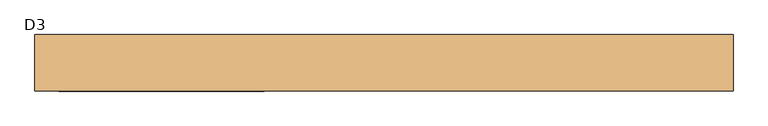
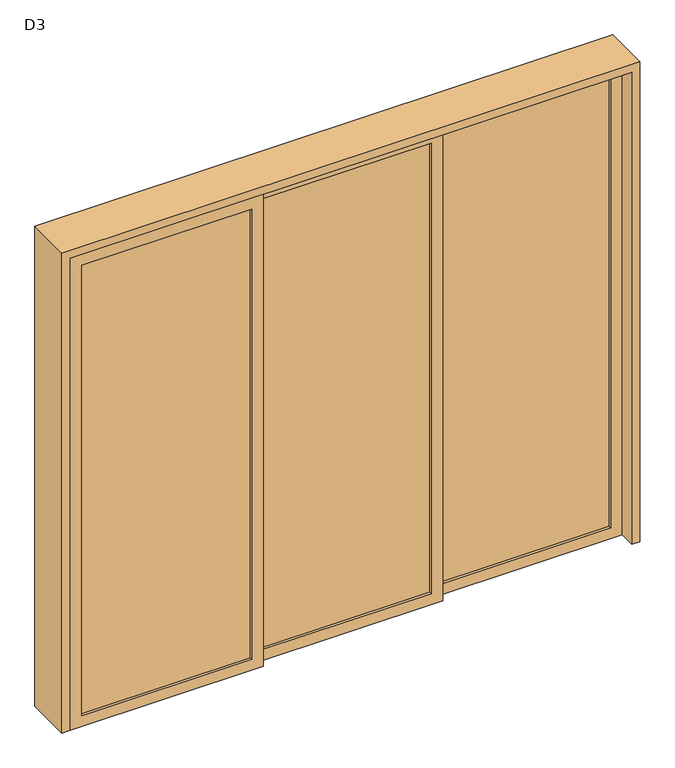
"""IFC4 building model written with IfcOpenShell, lengths in millimetres: door geometry, D3."""

from ifc_helpers import new_model, si_unit, frame, origin, place, context, project, spatial, polyline, outline, extrude, source, transform, mapped, element, save


def d3_d2ac5bf4(model_context):
    return source(origin(), model_context, "Body", "SweptSolid", [
        extrude(outline(polyline([(1380.7580012, -5.8333333), (1380.7580012, -19.1666667), (563.2580012, -19.1666667), (563.2580012, -5.8333333), (1380.7580012, -5.8333333)])), frame((0.0, 0.0, 55.0), z_axis=(0.0, 0.0, 1.0), x_axis=(1.0, 0.0, 0.0)), (0.0, 0.0, 1.0), 2290.0),
        extrude(outline(polyline([(0.0, 1435.7580012), (2400.0, 1435.7580012), (2400.0, 508.2580012), (0.0, 508.2580012), (0.0, 1435.7580012)]), holes=[polyline([(55.0, 1380.7580012), (55.0, 563.2580012), (2345.0, 563.2580012), (2345.0, 1380.7580012), (55.0, 1380.7580012)])]), frame((0.0, -32.5, 0.0), z_axis=(0.0, 1.0, 0.0), x_axis=(0.0, 0.0, 1.0)), (0.0, 0.0, 1.0), 40.0),
        extrude(outline(polyline([(494.9246679, -45.8333333), (494.9246679, -59.1666667), (-322.5753321, -59.1666667), (-322.5753321, -45.8333333), (494.9246679, -45.8333333)])), frame((0.0, 0.0, 55.0), z_axis=(0.0, 0.0, 1.0), x_axis=(1.0, 0.0, 0.0)), (0.0, 0.0, 1.0), 2290.0),
        extrude(outline(polyline([(0.0, 549.9246679), (2400.0, 549.9246679), (2400.0, -377.5753321), (0.0, -377.5753321), (0.0, 549.9246679)]), holes=[polyline([(55.0, 494.9246679), (55.0, -322.5753321), (2345.0, -322.5753321), (2345.0, 494.9246679), (55.0, 494.9246679)])]), frame((0.0, -72.5, 0.0), z_axis=(0.0, 1.0, 0.0), x_axis=(0.0, 0.0, 1.0)), (0.0, 0.0, 1.0), 40.0),
        extrude(outline(polyline([(-391.7419988, -85.8333333), (-391.7419988, -99.1666667), (-1209.2419988, -99.1666667), (-1209.2419988, -85.8333333), (-391.7419988, -85.8333333)])), frame((0.0, 0.0, 55.0), z_axis=(0.0, 0.0, 1.0), x_axis=(1.0, 0.0, 0.0)), (0.0, 0.0, 1.0), 2290.0),
        extrude(outline(polyline([(0.0, -336.7419988), (2400.0, -336.7419988), (2400.0, -1264.2419988), (0.0, -1264.2419988), (0.0, -336.7419988)]), holes=[polyline([(55.0, -391.7419988), (55.0, -1209.2419988), (2345.0, -1209.2419988), (2345.0, -391.7419988), (55.0, -391.7419988)])]), frame((0.0, -112.5, 0.0), z_axis=(0.0, 1.0, 0.0), x_axis=(0.0, 0.0, 1.0)), (0.0, 0.0, 1.0), 40.0),
        extrude(outline(polyline([(0.0, -1304.2419988), (0.0, -1264.2419988), (2400.0, -1264.2419988), (2400.0, 1435.7580012), (0.0, 1435.7580012), (0.0, 1475.7580012), (2440.0, 1475.7580012), (2440.0, -1304.2419988), (0.0, -1304.2419988)])), frame((0.0, -112.5, 0.0), z_axis=(0.0, 1.0, 0.0), x_axis=(0.0, 0.0, 1.0)), (0.0, 0.0, 1.0), 225.0),
    ])


if __name__ == "__main__":
    model = new_model("IFC4")
    model_context = context("Model", 3, world=origin())
    ifc_project = project(units=[si_unit("LENGTHUNIT", "METRE", prefix="MILLI")], contexts=[model_context])
    site = spatial("IfcSite", under=ifc_project)
    building = spatial("IfcBuilding", under=site)
    placement = place(None, origin())
    d3_shape = d3_d2ac5bf4(model_context)
    element("IfcDoor", 1, ObjectType="D3", at=placement, inside=building, context=model_context, shape_type="MappedRepresentation", body=[
        mapped(d3_shape, transform((0.0, 0.0, 0.0), x_axis=(1.0, 0.0, 0.0), y_axis=(0.0, 1.0, 0.0), z_axis=(0.0, 0.0, 1.0))),
    ])
    save(model, "model.ifc")

# Revit data of these elements
# Type "D3"
#   Type Mark = "52"
#   Operation = "UserDefined"
#   Width = 2700 mm
#   Thickness = 40 mm
#   Rough Width = 2780 mm
#   Rough Height = 2440 mm
#   Panel Width = 927.5 mm
#   Panel Frame = 55 mm
#   Height = 2400 mm
#   Frame Depth = 40 mm
#   Glass Material = Sliding Door Glass
#   Frame Material = Sliding Door Frame
#   Function = (empty or 0)
# Element 1 (IfcDoor, "D3")
#   Materials on its faces: "Sliding Door Frame", "Sliding Door Glass"
# Materials
#   "Sliding Door Glass": colour RGB 247 247 247, transparency 0.68
#   "Sliding Door Frame": colour RGB 160 107 8, transparency 0
